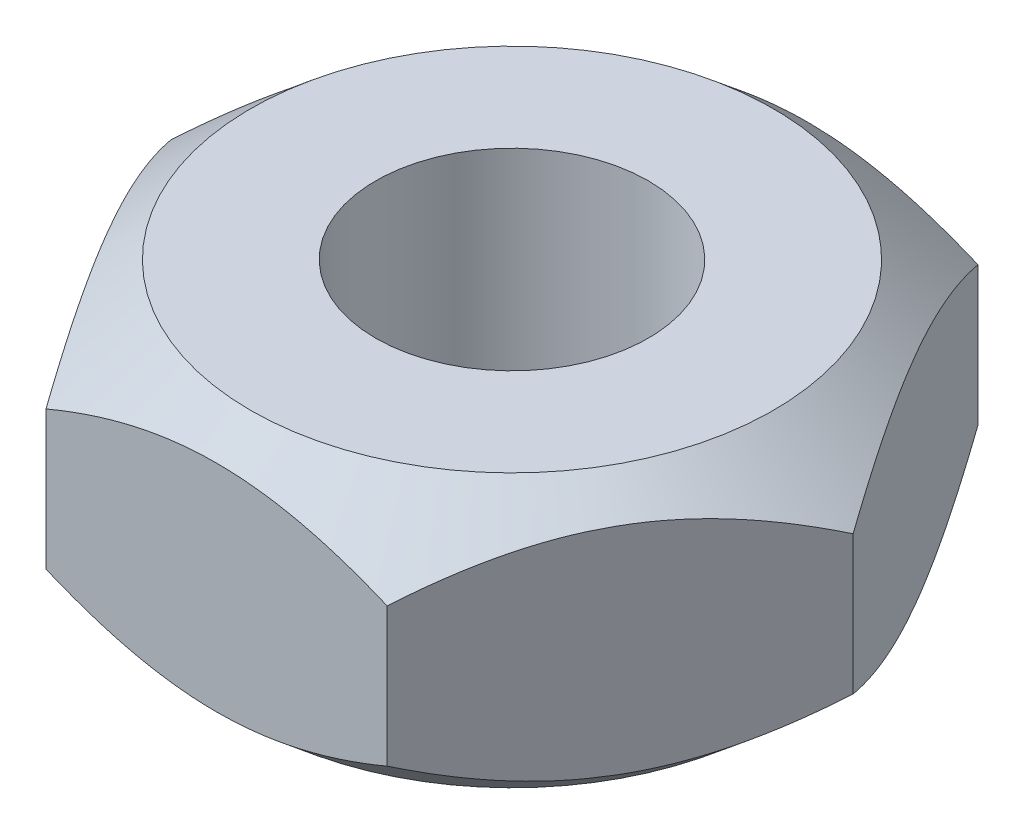
SolidWorks part; units mm, degrees
material "Plain Carbon Steel"
ref_plane "Front Plane" through (0, 0, 0) normal (0, 0, 1) x (1, 0, 0)
ref_plane "Top Plane" through (0, 0, 0) normal (0, 1, 0) x (1, 0, 0)
ref_plane "Right Plane" through (0, 0, 0) normal (1, 0, 0) x (0, 0, -1)
sketch "Hex Nut Profile" plane through (0, 0, 0) normal (0, 1, 0) x (1, 0, 0)
  line L1 (15.0111, 0) -> (7.5056, 13)
  line L2 (7.5056, 13) -> (-7.5056, 13)
  line L3 (-7.5056, 13) -> (-15.0111, 0)
  line L4 (-15.0111, 0) -> (-7.5056, -13)
  line L5 (-7.5056, -13) -> (7.5056, -13)
  line L6 (7.5056, -13) -> (15.0111, 0)
  circle A0 centre (0, 0) radius 13 construction
  circle A1 centre (0, 0) radius 6
  dimension "D2" = 12
  dimension "D1" = 26
extrude "Hex Nut Body" add sketch "Hex Nut Profile" along normal mid plane 12
sketch "Chamfer Circle Ø23" plane through (0, 6, 0) normal (0, 1, 0) x (1, 0, 0)
  circle A0 centre (0, 0) radius 11.5
  dimension "D1" = 23
extrude "Corner Chamfer 50°" cut sketch "Chamfer Circle Ø23" against normal through all draft 50 flip side to cut
mirror "Corner Chamfer Mirror" about plane through (0, 0, 0) normal (0, 1, 0) of "Corner Chamfer 50°"
